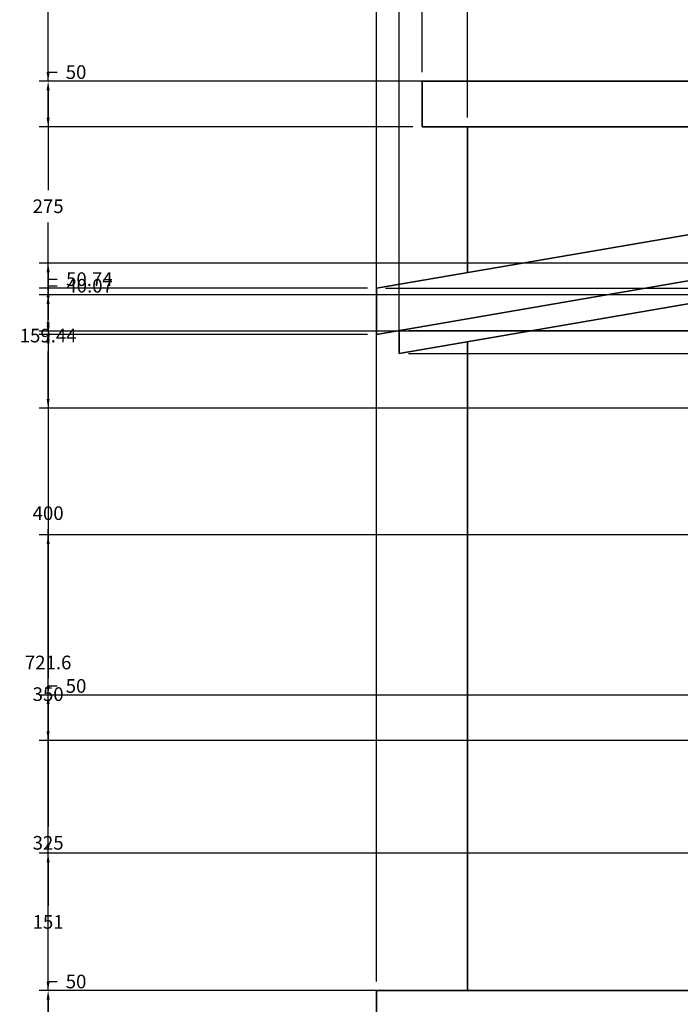
# Model space of a CAD drawing. Units: millimetres. Extents: x 937 to 4561, y 2711 to 5748.
# Tile 2 of 8: x 937 to 1663, y 4062 to 5145. Entities that reach past the tile are written whole.
import ezdxf

# ---------------------------------------------------------------- set-up
doc = ezdxf.new("R2010")
doc.units = ezdxf.units.MM
doc.header["$MEASUREMENT"] = 0
for name, color, linetype, lineweight in [('A-ANNO-DIMS', 2, 'Continuous', 18), ('A-ELEV', 7, 'Continuous', 35), ('A-ROOF', 1, 'Continuous', 35)]:
    doc.layers.add(name, color=color, linetype=linetype, lineweight=lineweight)
doc.styles.get("Standard").update_dxf_attribs({"font": 'arial.ttf'})
doc.dimstyles.get("Standard").update_dxf_attribs({"dimtxt": 15, "dimasz": 10, "dimexe": 10, "dimexo": 10, "dimgap": 10, "dimtad": 0, "dimtih": 1, "dimtoh": 1, "dimdec": 0, "dimzin": 0, "dimdsep": 46, "dimtxsty": 'Standard', "dimcen": 5, "dimadec": 0, "dimazin": 0, "dimtfac": 1, "dimtdec": 0, "dimtofl": 0, "dimtmove": 0, "dimatfit": 3, "dimfxl": 1, "dimtolj": 1, "dimtzin": 0, "dimarcsym": 0})

# ---------------------------------------------------------------- blocks, each defined once
blk = doc.blocks.new('*D15')
at = {"layer": 'A-ANNO-DIMS', "color": 0, "lineweight": -2, "transparency": 16777216}
for p, q in [((1329.5, 4086.9), (1329.5, 5747.9)), ((4179.5, 5586.9), (4179.5, 5747.9)), ((1339.5, 5737.9), (2722, 5737.9)), ((4169.5, 5737.9), (2787, 5737.9))]:
    blk.add_line(p, q, dxfattribs=at)
at = {"layer": 'A-ANNO-DIMS', "color": 0, "transparency": 16777216}
for points in [[(1339.5, 5739.6), (1339.5, 5736.2), (1329.5, 5737.9)], [(4169.5, 5739.6), (4169.5, 5736.2), (4179.5, 5737.9)]]:
    blk.add_solid(points, dxfattribs=at)
at = {"layer": 'Defpoints', "color": 0, "transparency": 16777216}
for p in [(4179.5, 5737.9), (4179.5, 5576.9), (1329.5, 4076.9)]:
    blk.add_point(p, dxfattribs=at)
at = {"layer": 'A-ANNO-DIMS', "color": 0, "transparency": 16777216, "insert": (2754.5, 5737.9), "char_height": 15, "attachment_point": 5}
blk.add_mtext('\\A1;2850', dxfattribs=at)
blk = doc.blocks.new('*D16')
at = {"layer": 'A-ANNO-DIMS', "color": 0, "lineweight": -2, "transparency": 16777216}
for p, q in [((1329.5, 4859.2), (1329.5, 5747.9)), ((2947.4, 5137.7), (2947.4, 5747.9)), ((1339.5, 5737.9), (2106.8, 5737.9)), ((2937.4, 5737.9), (2170.2, 5737.9))]:
    blk.add_line(p, q, dxfattribs=at)
at = {"layer": 'A-ANNO-DIMS', "color": 0, "transparency": 16777216}
for points in [[(1339.5, 5739.6), (1339.5, 5736.2), (1329.5, 5737.9)], [(2937.4, 5739.6), (2937.4, 5736.2), (2947.4, 5737.9)]]:
    blk.add_solid(points, dxfattribs=at)
at = {"layer": 'Defpoints', "color": 0, "transparency": 16777216}
for p in [(2947.4, 5737.9), (2947.4, 5127.7), (1329.5, 4849.2)]:
    blk.add_point(p, dxfattribs=at)
at = {"layer": 'A-ANNO-DIMS', "color": 0, "transparency": 16777216, "insert": (2138.5, 5737.9), "char_height": 15, "attachment_point": 5}
blk.add_mtext('\\A1;1618', dxfattribs=at)
blk = doc.blocks.new('*D20')
at = {"layer": 'A-ANNO-DIMS', "color": 0, "lineweight": -2, "transparency": 16777216}
for p, q in [((1379.5, 5086.9), (1379.5, 5747.9)), ((1429.5, 5036.9), (1429.5, 5747.9)), ((1369.5, 5737.9), (1359.5, 5737.9)), ((1439.5, 5737.9), (1449.5, 5737.9))]:
    blk.add_line(p, q, dxfattribs=at)
at = {"layer": 'A-ANNO-DIMS', "color": 0, "transparency": 16777216}
for points in [[(1369.5, 5739.6), (1369.5, 5736.2), (1379.5, 5737.9)], [(1439.5, 5739.6), (1439.5, 5736.2), (1429.5, 5737.9)]]:
    blk.add_solid(points, dxfattribs=at)
at = {"layer": 'Defpoints', "color": 0, "transparency": 16777216}
for p in [(1429.5, 5737.9), (1379.5, 5076.9), (1429.5, 5026.9)]:
    blk.add_point(p, dxfattribs=at)
at = {"layer": 'A-ANNO-DIMS', "color": 0, "transparency": 16777216, "insert": (1404.5, 5737.9), "char_height": 15, "attachment_point": 5}
blk.add_mtext('\\A1;50', dxfattribs=at)
blk = doc.blocks.new('*D21')
at = {"layer": 'A-ANNO-DIMS', "color": 0, "lineweight": -2, "transparency": 16777216}
for p, q in [((1329.5, 4808.5), (1329.5, 5747.9)), ((1354.5, 4787.4), (1354.5, 5747.9)), ((1319.5, 5737.9), (1309.5, 5737.9)), ((1364.5, 5737.9), (1374.5, 5737.9))]:
    blk.add_line(p, q, dxfattribs=at)
at = {"layer": 'A-ANNO-DIMS', "color": 0, "transparency": 16777216}
for points in [[(1319.5, 5739.6), (1319.5, 5736.2), (1329.5, 5737.9)], [(1364.5, 5739.6), (1364.5, 5736.2), (1354.5, 5737.9)]]:
    blk.add_solid(points, dxfattribs=at)
at = {"layer": 'Defpoints', "color": 0, "transparency": 16777216}
for p in [(1354.5, 5737.9), (1329.5, 4798.5), (1354.5, 4777.4)]:
    blk.add_point(p, dxfattribs=at)
at = {"layer": 'A-ANNO-DIMS', "color": 0, "transparency": 16777216, "insert": (1395.4, 5737.9), "char_height": 15, "attachment_point": 5}
blk.add_mtext('\\A1;25', dxfattribs=at)
blk = doc.blocks.new('*D43')
at = {"layer": 'A-ANNO-DIMS', "color": 0, "lineweight": -2, "transparency": 16777216}
for p, q in [((1329.5, 4086.9), (1329.5, 5747.9)), ((2579.5, 4086.9), (2579.5, 5747.9)), ((1339.5, 5737.9), (1922.8, 5737.9)), ((2569.5, 5737.9), (1986.2, 5737.9))]:
    blk.add_line(p, q, dxfattribs=at)
at = {"layer": 'A-ANNO-DIMS', "color": 0, "transparency": 16777216}
for points in [[(1339.5, 5739.6), (1339.5, 5736.2), (1329.5, 5737.9)], [(2569.5, 5739.6), (2569.5, 5736.2), (2579.5, 5737.9)]]:
    blk.add_solid(points, dxfattribs=at)
at = {"layer": 'Defpoints', "color": 0, "transparency": 16777216}
for p in [(2579.5, 5737.9), (1329.5, 4076.9), (2579.5, 4076.9)]:
    blk.add_point(p, dxfattribs=at)
at = {"layer": 'A-ANNO-DIMS', "color": 0, "transparency": 16777216, "insert": (1954.5, 5737.9), "char_height": 15, "attachment_point": 5}
blk.add_mtext('\\A1;1250', dxfattribs=at)
blk = doc.blocks.new('*D59')
at = {"layer": 'A-ANNO-DIMS', "color": 0, "lineweight": -2, "transparency": 16777216}
for p, q in [((1419.5, 4076.9), (958.5, 4076.9)), ((968.5, 4066.9), (968.5, 4019.6)), ((968.5, 3936.9), (968.5, 3984.2)), ((1419.5, 3926.9), (958.5, 3926.9))]:
    blk.add_line(p, q, dxfattribs=at)
at = {"layer": 'A-ANNO-DIMS', "color": 0, "transparency": 16777216}
for points in [[(966.8, 4066.9), (970.2, 4066.9), (968.5, 4076.9)], [(966.8, 3936.9), (970.2, 3936.9), (968.5, 3926.9)]]:
    blk.add_solid(points, dxfattribs=at)
at = {"layer": 'Defpoints', "color": 0, "transparency": 16777216}
for p in [(968.5, 4076.9), (1429.5, 4076.9), (1429.5, 3926.9)]:
    blk.add_point(p, dxfattribs=at)
at = {"layer": 'A-ANNO-DIMS', "color": 0, "transparency": 16777216, "insert": (968.5, 4001.9), "char_height": 15, "attachment_point": 5}
blk.add_mtext('\\A1;150', dxfattribs=at)
blk = doc.blocks.new('*D60')
at = {"layer": 'A-ANNO-DIMS', "color": 0, "lineweight": -2, "transparency": 16777216}
for p, q in [((1784.5, 4401.9), (958.5, 4401.9)), ((968.5, 4391.9), (968.5, 4257.1)), ((968.5, 4086.9), (968.5, 4221.7)), ((1419.5, 4076.9), (958.5, 4076.9))]:
    blk.add_line(p, q, dxfattribs=at)
at = {"layer": 'A-ANNO-DIMS', "color": 0, "transparency": 16777216}
for points in [[(966.8, 4391.9), (970.2, 4391.9), (968.5, 4401.9)], [(966.8, 4086.9), (970.2, 4086.9), (968.5, 4076.9)]]:
    blk.add_solid(points, dxfattribs=at)
at = {"layer": 'Defpoints', "color": 0, "transparency": 16777216}
for p in [(968.5, 4401.9), (1794.5, 4401.9), (1429.5, 4076.9)]:
    blk.add_point(p, dxfattribs=at)
at = {"layer": 'A-ANNO-DIMS', "color": 0, "transparency": 16777216, "insert": (968.5, 4239.4), "char_height": 15, "attachment_point": 5}
blk.add_mtext('\\A1;325', dxfattribs=at)
blk = doc.blocks.new('*D61')
at = {"layer": 'A-ANNO-DIMS', "color": 0, "lineweight": -2, "transparency": 16777216}
for p, q in [((1784.5, 4801.9), (958.5, 4801.9)), ((968.5, 4791.9), (968.5, 4619.6)), ((968.5, 4411.9), (968.5, 4584.2)), ((1784.5, 4401.9), (958.5, 4401.9))]:
    blk.add_line(p, q, dxfattribs=at)
at = {"layer": 'A-ANNO-DIMS', "color": 0, "transparency": 16777216}
for points in [[(966.8, 4791.9), (970.2, 4791.9), (968.5, 4801.9)], [(966.8, 4411.9), (970.2, 4411.9), (968.5, 4401.9)]]:
    blk.add_solid(points, dxfattribs=at)
at = {"layer": 'Defpoints', "color": 0, "transparency": 16777216}
for p in [(968.5, 4801.9), (1794.5, 4801.9), (1794.5, 4401.9)]:
    blk.add_point(p, dxfattribs=at)
at = {"layer": 'A-ANNO-DIMS', "color": 0, "transparency": 16777216, "insert": (968.5, 4601.9), "char_height": 15, "attachment_point": 5}
blk.add_mtext('\\A1;400', dxfattribs=at)
blk = doc.blocks.new('*D62')
at = {"layer": 'A-ANNO-DIMS', "color": 0, "lineweight": -2, "transparency": 16777216}
for p, q in [((1419.5, 5076.9), (958.5, 5076.9)), ((968.5, 5066.9), (968.5, 4957.1)), ((968.5, 4811.9), (968.5, 4921.7)), ((1784.5, 4801.9), (958.5, 4801.9))]:
    blk.add_line(p, q, dxfattribs=at)
at = {"layer": 'A-ANNO-DIMS', "color": 0, "transparency": 16777216}
for points in [[(966.8, 5066.9), (970.2, 5066.9), (968.5, 5076.9)], [(966.8, 4811.9), (970.2, 4811.9), (968.5, 4801.9)]]:
    blk.add_solid(points, dxfattribs=at)
at = {"layer": 'Defpoints', "color": 0, "transparency": 16777216}
for p in [(968.5, 5076.9), (1429.5, 5076.9), (1794.5, 4801.9)]:
    blk.add_point(p, dxfattribs=at)
at = {"layer": 'A-ANNO-DIMS', "color": 0, "transparency": 16777216, "insert": (968.5, 4939.4), "char_height": 15, "attachment_point": 5}
blk.add_mtext('\\A1;275', dxfattribs=at)
blk = doc.blocks.new('*D63')
at = {"layer": 'A-ANNO-DIMS', "color": 0, "lineweight": -2, "transparency": 16777216}
for p, q in [((3169.5, 5576.9), (958.5, 5576.9)), ((968.5, 5566.9), (968.5, 5344.6)), ((968.5, 5086.9), (968.5, 5309.2)), ((1419.5, 5076.9), (958.5, 5076.9))]:
    blk.add_line(p, q, dxfattribs=at)
at = {"layer": 'A-ANNO-DIMS', "color": 0, "transparency": 16777216}
for points in [[(966.8, 5566.9), (970.2, 5566.9), (968.5, 5576.9)], [(966.8, 5086.9), (970.2, 5086.9), (968.5, 5076.9)]]:
    blk.add_solid(points, dxfattribs=at)
at = {"layer": 'Defpoints', "color": 0, "transparency": 16777216}
for p in [(968.5, 5576.9), (3179.5, 5576.9), (1429.5, 5076.9)]:
    blk.add_point(p, dxfattribs=at)
at = {"layer": 'A-ANNO-DIMS', "color": 0, "transparency": 16777216, "insert": (968.5, 5326.9), "char_height": 15, "attachment_point": 5}
blk.add_mtext('\\A1;500', dxfattribs=at)
blk = doc.blocks.new('*D64')
at = {"layer": 'A-ANNO-DIMS', "color": 0, "lineweight": -2, "transparency": 16777216}
for p, q in [((968.5, 4076.9), (968.5, 4086.9)), ((968.5, 4086.9), (978.5, 4086.9)), ((1319.5, 4076.9), (958.5, 4076.9)), ((968.5, 4036.9), (968.5, 4066.9)), ((1319.5, 4026.9), (958.5, 4026.9))]:
    blk.add_line(p, q, dxfattribs=at)
at = {"layer": 'A-ANNO-DIMS', "color": 0, "transparency": 16777216}
for points in [[(966.8, 4066.9), (970.2, 4066.9), (968.5, 4076.9)], [(966.8, 4036.9), (970.2, 4036.9), (968.5, 4026.9)]]:
    blk.add_solid(points, dxfattribs=at)
at = {"layer": 'Defpoints', "color": 0, "transparency": 16777216}
for p in [(968.5, 4076.9), (1329.5, 4076.9), (1329.5, 4026.9)]:
    blk.add_point(p, dxfattribs=at)
at = {"layer": 'A-ANNO-DIMS', "color": 0, "transparency": 16777216, "insert": (999.2, 4086.9), "char_height": 15, "attachment_point": 5}
blk.add_mtext('\\A1;50', dxfattribs=at)
blk = doc.blocks.new('*D66')
at = {"layer": 'A-ANNO-DIMS', "color": 0, "lineweight": -2, "transparency": 16777216}
for p, q in [((968.5, 4849.2), (968.5, 4859.2)), ((968.5, 4859.2), (978.5, 4859.2)), ((1319.5, 4849.2), (958.5, 4849.2)), ((968.5, 4808.5), (968.5, 4839.2)), ((1319.5, 4798.5), (958.5, 4798.5))]:
    blk.add_line(p, q, dxfattribs=at)
at = {"layer": 'A-ANNO-DIMS', "color": 0, "transparency": 16777216}
for points in [[(966.8, 4839.2), (970.2, 4839.2), (968.5, 4849.2)], [(966.8, 4808.5), (970.2, 4808.5), (968.5, 4798.5)]]:
    blk.add_solid(points, dxfattribs=at)
at = {"layer": 'Defpoints', "color": 0, "transparency": 16777216}
for p in [(968.5, 4849.2), (1329.5, 4849.2), (1329.5, 4798.5)]:
    blk.add_point(p, dxfattribs=at)
at = {"layer": 'A-ANNO-DIMS', "color": 0, "transparency": 16777216, "insert": (1013.8, 4859.2), "char_height": 15, "attachment_point": 5}
blk.add_mtext('\\A1;50.74', dxfattribs=at)
blk = doc.blocks.new('*D67')
at = {"layer": 'A-ANNO-DIMS', "color": 0, "lineweight": -2, "transparency": 16777216}
for p, q in [((1319.5, 4798.5), (958.5, 4798.5)), ((968.5, 4788.5), (968.5, 4455.4)), ((968.5, 4086.9), (968.5, 4420)), ((1319.5, 4076.9), (958.5, 4076.9))]:
    blk.add_line(p, q, dxfattribs=at)
at = {"layer": 'A-ANNO-DIMS', "color": 0, "transparency": 16777216}
for points in [[(966.8, 4788.5), (970.2, 4788.5), (968.5, 4798.5)], [(966.8, 4086.9), (970.2, 4086.9), (968.5, 4076.9)]]:
    blk.add_solid(points, dxfattribs=at)
at = {"layer": 'Defpoints', "color": 0, "transparency": 16777216}
for p in [(968.5, 4798.5), (1329.5, 4798.5), (1329.5, 4076.9)]:
    blk.add_point(p, dxfattribs=at)
at = {"layer": 'A-ANNO-DIMS', "color": 0, "transparency": 16777216, "insert": (968.5, 4437.7), "char_height": 15, "attachment_point": 5}
blk.add_mtext('\\A1;721.6', dxfattribs=at)
blk = doc.blocks.new('*D68')
at = {"layer": 'A-ANNO-DIMS', "color": 0, "lineweight": -2, "transparency": 16777216}
for p, q in [((4490.5, 4812.8), (4490.5, 4822.8)), ((4490.5, 4822.8), (4500.5, 4822.8)), ((1364.5, 4802.8), (4500.5, 4802.8)), ((1364.5, 4777.4), (4500.5, 4777.4)), ((4490.5, 4767.4), (4490.5, 4757.4))]:
    blk.add_line(p, q, dxfattribs=at)
at = {"layer": 'A-ANNO-DIMS', "color": 0, "transparency": 16777216}
for points in [[(4488.8, 4812.8), (4492.2, 4812.8), (4490.5, 4802.8)], [(4488.8, 4767.4), (4492.2, 4767.4), (4490.5, 4777.4)]]:
    blk.add_solid(points, dxfattribs=at)
at = {"layer": 'Defpoints', "color": 0, "transparency": 16777216}
for p in [(1354.5, 4802.8), (4490.5, 4802.8), (1354.5, 4777.4)]:
    blk.add_point(p, dxfattribs=at)
at = {"layer": 'A-ANNO-DIMS', "color": 0, "transparency": 16777216, "insert": (4535.9, 4822.8), "char_height": 15, "attachment_point": 5}
blk.add_mtext('\\A1;25.37', dxfattribs=at)
blk = doc.blocks.new('*D69')
at = {"layer": 'A-ANNO-DIMS', "color": 0, "lineweight": -2, "transparency": 16777216}
for p, q in [((2957.4, 5127.7), (4500.5, 5127.7)), ((4490.5, 5117.7), (4490.5, 5006.1)), ((4490.5, 4859.2), (4490.5, 4970.8)), ((1339.5, 4849.2), (4500.5, 4849.2))]:
    blk.add_line(p, q, dxfattribs=at)
at = {"layer": 'A-ANNO-DIMS', "color": 0, "transparency": 16777216}
for points in [[(4488.8, 5117.7), (4492.2, 5117.7), (4490.5, 5127.7)], [(4488.8, 4859.2), (4492.2, 4859.2), (4490.5, 4849.2)]]:
    blk.add_solid(points, dxfattribs=at)
at = {"layer": 'Defpoints', "color": 0, "transparency": 16777216}
for p in [(2947.4, 5127.7), (4490.5, 5127.7), (1329.5, 4849.2)]:
    blk.add_point(p, dxfattribs=at)
at = {"layer": 'A-ANNO-DIMS', "color": 0, "transparency": 16777216, "insert": (4490.5, 4988.5), "char_height": 15, "attachment_point": 5}
blk.add_mtext('\\A1;278.45', dxfattribs=at)
blk = doc.blocks.new('*D70')
at = {"layer": 'A-ANNO-DIMS', "color": 0, "lineweight": -2, "transparency": 16777216}
for p, q in [((968.5, 5076.9), (968.5, 5086.9)), ((968.5, 5086.9), (978.5, 5086.9)), ((1369.5, 5076.9), (958.5, 5076.9)), ((968.5, 5036.9), (968.5, 5066.9)), ((1369.5, 5026.9), (958.5, 5026.9))]:
    blk.add_line(p, q, dxfattribs=at)
at = {"layer": 'A-ANNO-DIMS', "color": 0, "transparency": 16777216}
for points in [[(966.8, 5066.9), (970.2, 5066.9), (968.5, 5076.9)], [(966.8, 5036.9), (970.2, 5036.9), (968.5, 5026.9)]]:
    blk.add_solid(points, dxfattribs=at)
at = {"layer": 'Defpoints', "color": 0, "transparency": 16777216}
for p in [(968.5, 5076.9), (1379.5, 5076.9), (1379.5, 5026.9)]:
    blk.add_point(p, dxfattribs=at)
at = {"layer": 'A-ANNO-DIMS', "color": 0, "transparency": 16777216, "insert": (999.2, 5086.9), "char_height": 15, "attachment_point": 5}
blk.add_mtext('\\A1;50', dxfattribs=at)
blk = doc.blocks.new('*D74')
at = {"layer": 'A-ANNO-DIMS', "color": 0, "lineweight": -2, "transparency": 16777216}
for p, q in [((968.5, 4401.9), (968.5, 4411.9)), ((968.5, 4411.9), (978.5, 4411.9)), ((1719.5, 4401.9), (958.5, 4401.9)), ((968.5, 4361.9), (968.5, 4391.9)), ((1719.5, 4351.9), (958.5, 4351.9))]:
    blk.add_line(p, q, dxfattribs=at)
at = {"layer": 'A-ANNO-DIMS', "color": 0, "transparency": 16777216}
for points in [[(966.8, 4391.9), (970.2, 4391.9), (968.5, 4401.9)], [(966.8, 4361.9), (970.2, 4361.9), (968.5, 4351.9)]]:
    blk.add_solid(points, dxfattribs=at)
at = {"layer": 'Defpoints', "color": 0, "transparency": 16777216}
for p in [(968.5, 4401.9), (1729.5, 4401.9), (1729.5, 4351.9)]:
    blk.add_point(p, dxfattribs=at)
at = {"layer": 'A-ANNO-DIMS', "color": 0, "transparency": 16777216, "insert": (999.2, 4411.9), "char_height": 15, "attachment_point": 5}
blk.add_mtext('\\A1;50', dxfattribs=at)
blk = doc.blocks.new('*D77')
at = {"layer": 'A-ANNO-DIMS', "color": 0, "lineweight": -2, "transparency": 16777216}
for p, q in [((968.5, 4842), (968.5, 4852)), ((968.5, 4852), (978.5, 4852)), ((1719.5, 4842), (958.5, 4842)), ((968.5, 4811.9), (968.5, 4832)), ((1784.5, 4801.9), (958.5, 4801.9))]:
    blk.add_line(p, q, dxfattribs=at)
at = {"layer": 'A-ANNO-DIMS', "color": 0, "transparency": 16777216}
for points in [[(966.8, 4832), (970.2, 4832), (968.5, 4842)], [(966.8, 4811.9), (970.2, 4811.9), (968.5, 4801.9)]]:
    blk.add_solid(points, dxfattribs=at)
at = {"layer": 'Defpoints', "color": 0, "transparency": 16777216}
for p in [(968.5, 4842), (1729.5, 4842), (1794.5, 4801.9)]:
    blk.add_point(p, dxfattribs=at)
at = {"layer": 'A-ANNO-DIMS', "color": 0, "transparency": 16777216, "insert": (1014.1, 4852), "char_height": 15, "attachment_point": 5}
blk.add_mtext('\\A1;40.07', dxfattribs=at)
blk = doc.blocks.new('*D79')
at = {"layer": 'A-ANNO-DIMS', "color": 0, "lineweight": -2, "transparency": 16777216}
for p, q in [((3019.5, 4876.9), (958.5, 4876.9)), ((968.5, 4866.9), (968.5, 4814.8)), ((968.5, 4727.5), (968.5, 4779.5)), ((2569.5, 4717.5), (958.5, 4717.5))]:
    blk.add_line(p, q, dxfattribs=at)
at = {"layer": 'A-ANNO-DIMS', "color": 0, "transparency": 16777216}
for points in [[(966.8, 4866.9), (970.2, 4866.9), (968.5, 4876.9)], [(966.8, 4727.5), (970.2, 4727.5), (968.5, 4717.5)]]:
    blk.add_solid(points, dxfattribs=at)
at = {"layer": 'Defpoints', "color": 0, "transparency": 16777216}
for p in [(968.5, 4876.9), (3029.5, 4876.9), (2579.5, 4717.5)]:
    blk.add_point(p, dxfattribs=at)
at = {"layer": 'A-ANNO-DIMS', "color": 0, "transparency": 16777216, "insert": (968.5, 4797.2), "char_height": 15, "attachment_point": 5}
blk.add_mtext('\\A1;159.44', dxfattribs=at)
blk = doc.blocks.new('*D86')
at = {"layer": 'A-ANNO-DIMS', "color": 0, "lineweight": -2, "transparency": 16777216}
for p, q in [((968.5, 4076.9), (968.5, 4086.9)), ((968.5, 4086.9), (978.5, 4086.9)), ((2569.5, 4076.9), (958.5, 4076.9)), ((968.5, 4036.9), (968.5, 4066.9)), ((2569.5, 4026.9), (958.5, 4026.9))]:
    blk.add_line(p, q, dxfattribs=at)
at = {"layer": 'A-ANNO-DIMS', "color": 0, "transparency": 16777216}
for points in [[(966.8, 4066.9), (970.2, 4066.9), (968.5, 4076.9)], [(966.8, 4036.9), (970.2, 4036.9), (968.5, 4026.9)]]:
    blk.add_solid(points, dxfattribs=at)
at = {"layer": 'Defpoints', "color": 0, "transparency": 16777216}
for p in [(968.5, 4076.9), (2579.5, 4076.9), (2579.5, 4026.9)]:
    blk.add_point(p, dxfattribs=at)
at = {"layer": 'A-ANNO-DIMS', "color": 0, "transparency": 16777216, "insert": (999.2, 4086.9), "char_height": 15, "attachment_point": 5}
blk.add_mtext('\\A1;50', dxfattribs=at)
blk = doc.blocks.new('*D87')
at = {"layer": 'A-ANNO-DIMS', "color": 0, "lineweight": -2, "transparency": 16777216}
for p, q in [((2794.5, 4227.9), (958.5, 4227.9)), ((968.5, 4217.9), (968.5, 4170.1)), ((968.5, 4086.9), (968.5, 4134.7)), ((2719.5, 4076.9), (958.5, 4076.9))]:
    blk.add_line(p, q, dxfattribs=at)
at = {"layer": 'A-ANNO-DIMS', "color": 0, "transparency": 16777216}
for points in [[(966.8, 4217.9), (970.2, 4217.9), (968.5, 4227.9)], [(966.8, 4086.9), (970.2, 4086.9), (968.5, 4076.9)]]:
    blk.add_solid(points, dxfattribs=at)
at = {"layer": 'Defpoints', "color": 0, "transparency": 16777216}
for p in [(968.5, 4227.9), (2804.5, 4227.9), (2729.5, 4076.9)]:
    blk.add_point(p, dxfattribs=at)
at = {"layer": 'A-ANNO-DIMS', "color": 0, "transparency": 16777216, "insert": (968.5, 4152.4), "char_height": 15, "attachment_point": 5}
blk.add_mtext('\\A1;151', dxfattribs=at)
blk = doc.blocks.new('*D93')
at = {"layer": 'A-ANNO-DIMS', "color": 0, "lineweight": -2, "transparency": 16777216}
for p, q in [((2794.5, 4577.9), (958.5, 4577.9)), ((968.5, 4567.9), (968.5, 4420.6)), ((968.5, 4237.9), (968.5, 4385.2)), ((2794.5, 4227.9), (958.5, 4227.9))]:
    blk.add_line(p, q, dxfattribs=at)
at = {"layer": 'A-ANNO-DIMS', "color": 0, "transparency": 16777216}
for points in [[(966.8, 4567.9), (970.2, 4567.9), (968.5, 4577.9)], [(966.8, 4237.9), (970.2, 4237.9), (968.5, 4227.9)]]:
    blk.add_solid(points, dxfattribs=at)
at = {"layer": 'Defpoints', "color": 0, "transparency": 16777216}
for p in [(968.5, 4577.9), (2804.5, 4577.9), (2804.5, 4227.9)]:
    blk.add_point(p, dxfattribs=at)
at = {"layer": 'A-ANNO-DIMS', "color": 0, "transparency": 16777216, "insert": (968.5, 4402.9), "char_height": 15, "attachment_point": 5}
blk.add_mtext('\\A1;350', dxfattribs=at)

msp = doc.modelspace()

# ---------------------------------------------------------------- linework, layer by layer
at = {"layer": 'A-ELEV'}
for p, q in [((1429.4852, 4866.4468), (1429.4852, 5026.9013)), ((1329.4852, 4798.5021), (1329.4852, 4849.2371)), ((1429.4852, 4076.9013), (1429.4852, 4790.3443)), ((1429.4852, 4076.9013), (1329.4852, 4076.9013)), ((1329.4852, 4076.9013), (1329.4852, 4026.9013)), ((1429.4852, 4076.9013), (3479.4852, 4076.9013))]:
    msp.add_line(p, q, dxfattribs=at)
at = {"layer": 'A-ROOF'}
for p, q in [((2947.4456, 5127.6834), (1329.4852, 4849.2371)), ((2947.1723, 5076.9013), (1329.4852, 4798.5021)), ((1379.4852, 5026.9013), (1379.4852, 5076.9013)), ((1379.4852, 5076.9013), (1429.4852, 5076.9013)), ((1429.4852, 5076.9013), (2652.3676, 5076.9013)), ((2922.0122, 5047.2038), (1354.4852, 4777.437)), ((1429.4852, 5026.9013), (1379.4852, 5026.9013)), ((1429.4852, 5026.9013), (2361.834, 5026.9013)), ((1354.4852, 4777.437), (1354.4852, 4802.8045))]:
    msp.add_line(p, q, dxfattribs=at)

# ---------------------------------------------------------------- dimensions: what is measured, and where the dimension line sits
at = {"layer": 'A-ANNO-DIMS'}
for base, p1, p2, picture, middle in [((1354.4852, 5737.9013), (1329.4852, 4798.5021), (1354.4852, 4777.437), '*D21', (1395.4129, 5737.9013)), ((4179.4852, 5737.9013), (1329.4852, 4076.9013), (4179.4852, 5576.9013), '*D15', (2754.4852, 5737.9013)), ((2947.4456, 5737.9013), (1329.4852, 4849.2371), (2947.4456, 5127.6834), '*D16', (2138.4654, 5737.9013)), ((2579.4852, 5737.9013), (1329.4852, 4076.9013), (2579.4852, 4076.9013), '*D43', (1954.4852, 5737.9013)), ((1429.4852, 5737.9013), (1379.4852, 5076.9013), (1429.4852, 5026.9013), '*D20', (1404.4852, 5737.9013))]:
    dim = msp.add_linear_dim(base=base, p1=p1, p2=p2, dimstyle='Standard', override={"dimdec": 0, "dimlfac": 1, "dimrnd": 0, "dimzin": 0, "dimdsep": 46, "dimlunit": 2}, dxfattribs=at)
    dim.commit()
    dim.dimension.update_dxf_attribs({"geometry": picture, "text_midpoint": middle})
for base, p1, p2, override, picture, middle in [((968.4852, 5576.9013), (1429.4852, 5076.9013), (3179.4852, 5576.9013), {"dimdec": 0, "dimlfac": 1, "dimrnd": 0, "dimzin": 0, "dimdsep": 46, "dimlunit": 2}, '*D63', (968.4852, 5326.9013)), ((4490.4852, 5127.6834), (1329.4852, 4849.2371), (2947.4456, 5127.6834), {"dimdec": 2, "dimlfac": 1, "dimrnd": 0, "dimzin": 0, "dimdsep": 46, "dimlunit": 2}, '*D69', (4490.4852, 4988.4602)), ((968.4852, 5076.9013), (1379.4852, 5026.9013), (1379.4852, 5076.9013), {"dimdec": 0, "dimlfac": 1, "dimrnd": 0, "dimzin": 0, "dimdsep": 46, "dimlunit": 2}, '*D70', (999.2031, 5086.9013)), ((968.4852, 5076.9013), (1794.4852, 4801.9013), (1429.4852, 5076.9013), {"dimdec": 0, "dimlfac": 1, "dimrnd": 0, "dimzin": 0, "dimdsep": 46, "dimlunit": 2}, '*D62', (968.4852, 4939.4013)), ((968.4852, 4876.9013), (2579.4852, 4717.4604), (3029.4852, 4876.9013), {"dimdec": 2, "dimlfac": 1, "dimrnd": 0, "dimzin": 0, "dimdsep": 46, "dimlunit": 2}, '*D79', (968.4852, 4797.1808)), ((968.4852, 4849.23711), (1329.4852, 4798.50208), (1329.4852, 4849.23711), {"dimdec": 2, "dimlfac": 1, "dimrnd": 0, "dimzin": 0, "dimdsep": 46, "dimlunit": 2}, '*D66', (1013.76317, 4859.23711)), ((968.4852, 4841.9734), (1794.4852, 4801.9013), (1729.4852, 4841.9734), {"dimdec": 2, "dimlfac": 1, "dimrnd": 0, "dimzin": 0, "dimdsep": 46, "dimlunit": 2}, '*D77', (1014.0957, 4851.9734)), ((4490.4852, 4802.8045), (1354.4852, 4777.437), (1354.4852, 4802.8045), {"dimdec": 2, "dimlfac": 1, "dimrnd": 0, "dimzin": 0, "dimdsep": 46, "dimlunit": 2}, '*D68', (4535.9218, 4822.8045)), ((968.4852, 4798.5021), (1329.4852, 4076.9013), (1329.4852, 4798.5021), {"dimdec": 1, "dimlfac": 1, "dimrnd": 0, "dimzin": 0, "dimdsep": 46, "dimlunit": 2}, '*D67', (968.4852, 4437.7017)), ((968.4852, 4801.9013), (1794.4852, 4401.9013), (1794.4852, 4801.9013), {"dimdec": 0, "dimlfac": 1, "dimrnd": 0, "dimzin": 0, "dimdsep": 46, "dimlunit": 2}, '*D61', (968.4852, 4601.9013)), ((968.4852, 4577.9047), (2804.4852, 4227.9047), (2804.4852, 4577.9047), {"dimdec": 0, "dimlfac": 1, "dimrnd": 0, "dimzin": 0, "dimdsep": 46, "dimlunit": 2}, '*D93', (968.4852, 4402.9047)), ((968.4852, 4401.9013), (1729.4852, 4351.9013), (1729.4852, 4401.9013), {"dimdec": 0, "dimlfac": 1, "dimrnd": 0, "dimzin": 0, "dimdsep": 46, "dimlunit": 2}, '*D74', (999.2031, 4411.9013)), ((968.4852, 4401.9013), (1429.4852, 4076.9013), (1794.4852, 4401.9013), {"dimdec": 0, "dimlfac": 1, "dimrnd": 0, "dimzin": 0, "dimdsep": 46, "dimlunit": 2}, '*D60', (968.4852, 4239.4013)), ((968.4852, 4227.9047), (2729.4852, 4076.9013), (2804.4852, 4227.9047), {"dimdec": 0, "dimlfac": 1, "dimrnd": 0, "dimzin": 0, "dimdsep": 46, "dimlunit": 2}, '*D87', (968.4852, 4152.403)), ((968.4852, 4076.9013), (1329.4852, 4026.9013), (1329.4852, 4076.9013), {"dimdec": 0, "dimlfac": 1, "dimrnd": 0, "dimzin": 0, "dimdsep": 46, "dimlunit": 2}, '*D64', (999.2031, 4086.9013)), ((968.4852, 4076.9013), (2579.4852, 4026.9013), (2579.4852, 4076.9013), {"dimdec": 0, "dimlfac": 1, "dimrnd": 0, "dimzin": 0, "dimdsep": 46, "dimlunit": 2}, '*D86', (999.2031, 4086.9013)), ((968.4852, 4076.9013), (1429.4852, 3926.9013), (1429.4852, 4076.9013), {"dimdec": 0, "dimlfac": 1, "dimrnd": 0, "dimzin": 0, "dimdsep": 46, "dimlunit": 2}, '*D59', (968.4852, 4001.9013))]:
    dim = msp.add_linear_dim(base=base, p1=p1, p2=p2, angle=90, dimstyle='Standard', override=override, dxfattribs=at)
    dim.commit()
    dim.dimension.update_dxf_attribs({"geometry": picture, "text_midpoint": middle})

doc.saveas('drawing.dxf')
